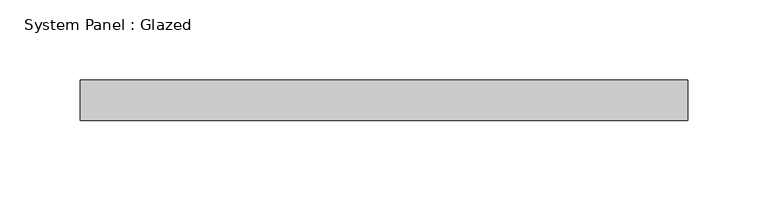
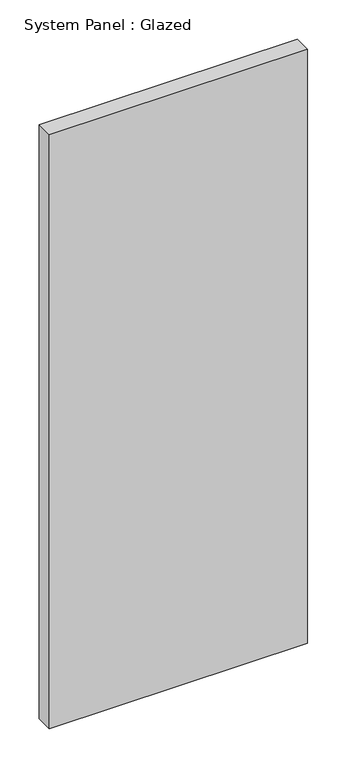
"""IFC4 building model written with IfcOpenShell, lengths in millimetres: plate geometry, System Panel : Glazed."""

from ifc_helpers import new_model, si_unit, origin, origin_with_axes, place, context, project, spatial, polyline, outline, extrude, source, transform, mapped, element, save


def system_panel_glazed_d518dbe9(model_context):
    return source(origin(), model_context, "Body", "SweptSolid", [
        extrude(outline(polyline([(189.4416667, 19.05), (-189.4416667, 19.05), (-189.4416667, 44.45), (189.4416667, 44.45), (189.4416667, 19.05)])), origin_with_axes(), (0.0, 0.0, 1.0), 920.75),
    ])


if __name__ == "__main__":
    model = new_model("IFC4")
    model_context = context("Model", 3, world=origin())
    ifc_project = project(units=[si_unit("LENGTHUNIT", "METRE", prefix="MILLI")], contexts=[model_context])
    site = spatial("IfcSite", under=ifc_project)
    building = spatial("IfcBuilding", under=site)
    placement = place(None, origin())
    system_panel_glazed_shape = system_panel_glazed_d518dbe9(model_context)
    element("IfcPlate", 1, ObjectType="System Panel : Glazed", at=placement, inside=building, context=model_context, shape_type="MappedRepresentation", body=[
        mapped(system_panel_glazed_shape, transform((0.0, 0.0, 0.0), x_axis=(1.0, 0.0, 0.0), y_axis=(0.0, 1.0, 0.0), z_axis=(0.0, 0.0, 1.0))),
    ])
    save(model, "model.ifc")

# Revit data of these elements
# Type "System Panel : Glazed"
#   Construction Type Id = "GSP4R"
#   Analytic Construction = "1/8 in Pilkington single glazing"
#   Visual Light Transmittance = 0.9
#   Solar Heat Gain Coefficient = 0.86
#   Heat Transfer Coefficient (U) = 1.18115 BTU/(h·ft²·°F)
#   Define Thermal Properties by = 1
# Element 1 (IfcPlate, "System Panel : Glazed")
#   Materials on its faces: "Glass"
# Materials
#   "Glass": class "Glass", colour RGB 0 128 192, transparency 0.75, Description = "Soda Lime Glass", Cost = 0
